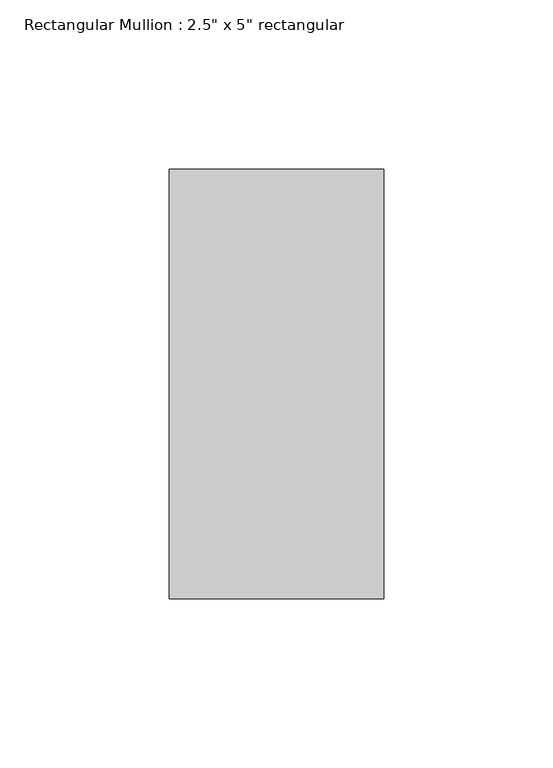
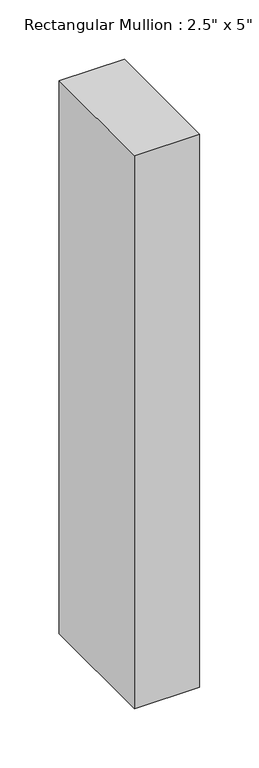
"""IFC4 building model written with IfcOpenShell, lengths in millimetres: member geometry."""

from ifc_helpers import new_model, si_unit, frame, origin, place, context, project, spatial, polyline, outline, extrude, source, transform, mapped, element, save


def member_ab4f2237(model_context):
    return source(origin(), model_context, "Body", "SweptSolid", [
        extrude(outline(polyline([(0.0, 63.5), (0.0, -63.5), (-63.5, -63.5), (-63.5, 63.5), (0.0, 63.5)])), frame((0.0, 0.0, -568.96), z_axis=(0.0, 0.0, 1.0), x_axis=(1.0, 0.0, 0.0)), (0.0, 0.0, 1.0), 568.96),
    ])


if __name__ == "__main__":
    model = new_model("IFC4")
    model_context = context("Model", 3, world=origin())
    ifc_project = project(units=[si_unit("LENGTHUNIT", "METRE", prefix="MILLI")], contexts=[model_context])
    site = spatial("IfcSite", under=ifc_project)
    building = spatial("IfcBuilding", under=site)
    placement = place(None, origin())
    member_shape = member_ab4f2237(model_context)
    element("IfcMember", 1, ObjectType="Rectangular Mullion : 2.5\" x 5\" rectangular", at=placement, inside=building, context=model_context, shape_type="MappedRepresentation", body=[
        mapped(member_shape, transform((0.0, 0.0, 0.0), x_axis=(1.0, 0.0, 0.0), y_axis=(0.0, 1.0, 0.0), z_axis=(0.0, 0.0, 1.0))),
    ])
    save(model, "model.ifc")

# Revit data of these elements
# Type "Rectangular Mullion : 2.5\" x 5\" rectangular"
#   built-in parameter 1007304 = 0.416667 (stored number, unit not read)
#   built-in parameter 1007301 = 0.104167 (stored number, unit not read)
#   built-in parameter 1007300 = 0.104167 (stored number, unit not read)
# Element 1 (IfcMember, "Rectangular Mullion : 2.5\" x 5\" rectangular")
#   Materials on its faces: "Aluminum"
# Materials
#   "Aluminum": class "Metal", colour RGB 247 247 247, transparency 0, Description = "Aluminum 6061", Cost = 0
